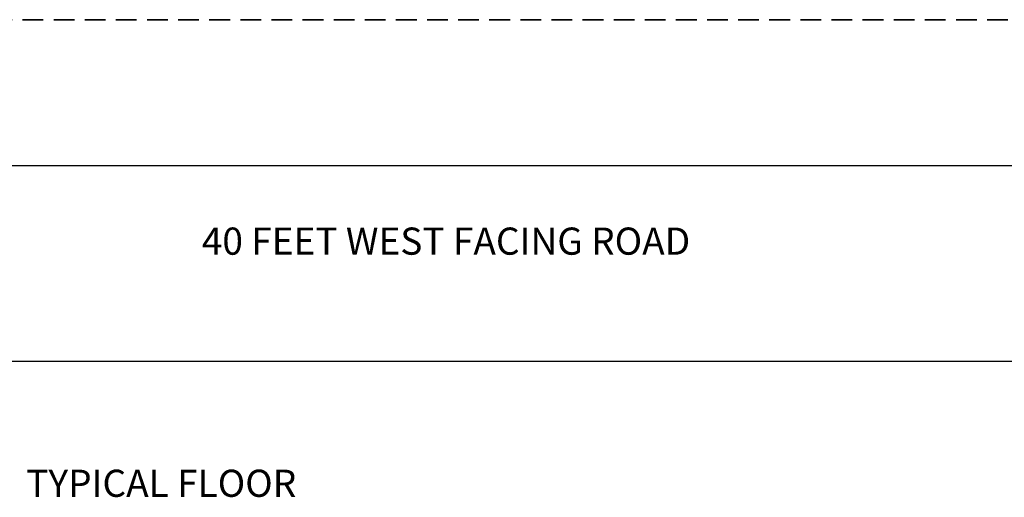
# Model space of a CAD drawing. Units: inches. Extents: x -7 to 1228, y -146 to 1091.
# Tile 19 of 88: x 513 to 815, y -146 to 0. Entities that reach past the tile are written whole.
import ezdxf

# ---------------------------------------------------------------- set-up
doc = ezdxf.new("R2010")
doc.units = ezdxf.units.IN
doc.linetypes.add('DASHED2', pattern=[9.525, 6.35, -3.175])
for name, color, linetype, lineweight in [('A-ANNO-TEXT', 7, 'Continuous', 18), ('C-PROP', 1, 'DASHED2', 35), ('C-ROAD', 7, 'Continuous', 25)]:
    doc.layers.add(name, color=color, linetype=linetype, lineweight=lineweight)
doc.styles.get("Standard").update_dxf_attribs({"font": 'arial.ttf'})

msp = doc.modelspace()

# ---------------------------------------------------------------- linework, layer by layer
at = {"layer": 'C-PROP'}
msp.add_line((0, 0), (1187, 0), dxfattribs=at)
at = {"layer": 'C-ROAD'}
for p, q in [((0, -44.69), (1187, -44.69)), ((0, -104.69), (1187, -104.69))]:
    msp.add_line(p, q, dxfattribs=at)

# ---------------------------------------------------------------- texts
at = {"layer": 'A-ANNO-TEXT', "char_height": 8.3203, "attachment_point": 1}
for s, insert in [('40 FEET WEST FACING ROAD', (569.21, -63.7)), ('{TYPICAL FLOOR}', (515.47, -137.9))]:
    msp.add_mtext_dynamic_manual_height_columns(s, width=225.8822, gutter_width=41.6, heights=[0], dxfattribs=dict(at, insert=insert))

doc.saveas('drawing.dxf')
